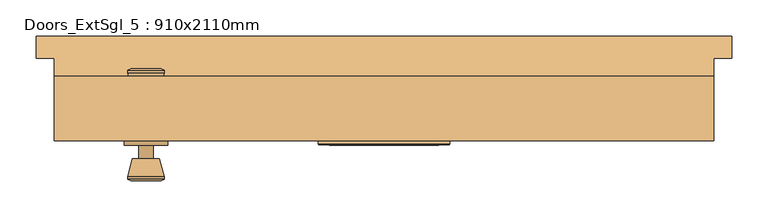
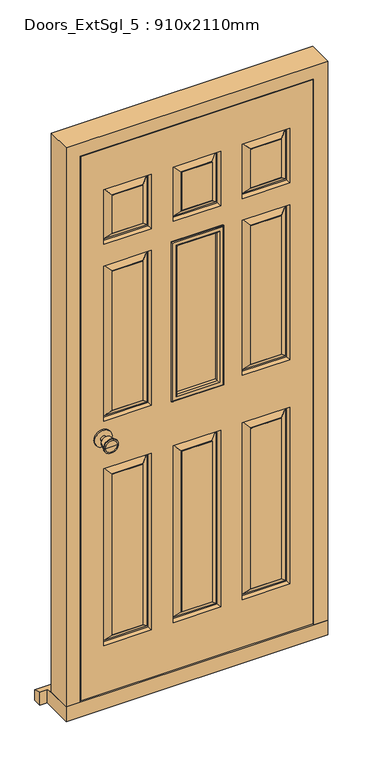
"""IFC4 building model written with IfcOpenShell, lengths in millimetres: door geometry, Doors_ExtSgl_5 : 910x2110mm."""

from ifc_helpers import new_model, si_unit, point, frame, frame_2d, origin, place, context, project, spatial, polyline, circle_curve, ellipse_curve, trimmed, segment, composite_curve, outline, extrude, faceted_brep, source, transform, mapped, element, save
from ifc_brep_helpers import plane_surface, cylinder_surface, revolved_surface, advanced_brep


def doors_extsgl_5_910x2110mm_d3ca6061(model_context):
    return source(origin(), model_context, "Body", "SolidModel", [
        advanced_brep(
        [(-328.4666667, -18.4, 1000.0), (-318.4666667, -18.4, 1000.0), (-338.4666667, -18.4, 1000.0), (-307.9907991, -67.4, 1000.0), (-328.4666667, -67.4, 1000.0), (-348.9425342, -67.4, 1000.0), (-303.4666667, -65.5721319, 1000.0), (-353.4666667, -65.5721319, 1000.0), (-303.4666667, -62.1084537, 1000.0), (-353.4666667, -62.1084537, 1000.0), (-309.8304306, -37.4, 1000.0), (-347.1029027, -37.4, 1000.0), (-318.4666667, -37.4, 1000.0), (-338.4666667, -37.4, 1000.0)],
        [
            (0, 1),
            (1, 2, circle_curve(frame((-328.4666667, -18.4, 1000.0), z_axis=(0.0, 1.0, 0.0), x_axis=(-1.0, 0.0, 0.0)), 10.0)),
            (2, 0),
            (2, 1, circle_curve(frame((-328.4666667, -18.4, 1000.0), z_axis=(0.0, 1.0, 0.0), x_axis=(-1.0, 0.0, 0.0)), 10.0)),
            (3, 4),
            (4, 5),
            (5, 3, circle_curve(frame((-328.4666667, -67.4, 1000.0), z_axis=(0.0, -1.0, 0.0), x_axis=(-1.0, 0.0, 0.0)), 20.4758676)),
            (3, 5, circle_curve(frame((-328.4666667, -67.4, 1000.0), z_axis=(0.0, -1.0, 0.0), x_axis=(-1.0, 0.0, 0.0)), 20.4758676)),
            (6, 3),
            (5, 7),
            (7, 6, circle_curve(frame((-328.4666667, -65.5721319, 1000.0), z_axis=(0.0, -1.0, 0.0), x_axis=(-1.0, 0.0, 0.0)), 25.0)),
            (6, 7, circle_curve(frame((-328.4666667, -65.5721319, 1000.0), z_axis=(0.0, -1.0, 0.0), x_axis=(-1.0, 0.0, 0.0)), 25.0)),
            (8, 6),
            (7, 9),
            (9, 8, circle_curve(frame((-328.4666667, -62.1084537, 1000.0), z_axis=(0.0, -1.0, 0.0), x_axis=(-1.0, 0.0, 0.0)), 25.0)),
            (8, 9, circle_curve(frame((-328.4666667, -62.1084537, 1000.0), z_axis=(0.0, -1.0, 0.0), x_axis=(-1.0, 0.0, 0.0)), 25.0)),
            (10, 8),
            (9, 11),
            (11, 10, circle_curve(frame((-328.4666667, -37.4, 1000.0), z_axis=(0.0, -1.0, 0.0), x_axis=(-1.0, 0.0, 0.0)), 18.636236)),
            (10, 11, circle_curve(frame((-328.4666667, -37.4, 1000.0), z_axis=(0.0, -1.0, 0.0), x_axis=(-1.0, 0.0, 0.0)), 18.636236)),
            (12, 10),
            (11, 13),
            (13, 12, circle_curve(frame((-328.4666667, -37.4, 1000.0), z_axis=(0.0, -1.0, 0.0), x_axis=(-1.0, 0.0, 0.0)), 10.0)),
            (12, 13, circle_curve(frame((-328.4666667, -37.4, 1000.0), z_axis=(0.0, -1.0, 0.0), x_axis=(-1.0, 0.0, 0.0)), 10.0)),
            (1, 12),
            (13, 2),
        ],
        [
            plane_surface(frame((-328.4666667, -18.4, 1000.0), z_axis=(0.0, 1.0, 0.0), x_axis=(-1.0, 0.0, 0.0))),
            plane_surface(frame((-328.4666667, -67.4, 1000.0), z_axis=(0.0, -1.0, 0.0), x_axis=(-1.0, 0.0, 0.0))),
            revolved_surface(polyline([(-348.9425342, -67.4, 1000.0), (-353.4666667, -65.5721319, 1000.0)]), (-328.4666667, -18.4, 1000.0), (0.0, 1.0, 0.0)),
            cylinder_surface(frame((-328.4666667, -18.4, 1000.0), z_axis=(0.0, 1.0, 0.0), x_axis=(-1.0, 0.0, 0.0)), 25.0),
            revolved_surface(polyline([(-353.4666667, -62.1084537, 1000.0), (-347.1029027, -37.4, 1000.0)]), (-328.4666667, -18.4, 1000.0), (0.0, 1.0, 0.0)),
            plane_surface(frame((-328.4666667, -37.4, 1000.0), z_axis=(0.0, 1.0, 0.0), x_axis=(-1.0, 0.0, 0.0))),
            cylinder_surface(frame((-328.4666667, -18.4, 1000.0), z_axis=(0.0, 1.0, 0.0), x_axis=(-1.0, 0.0, 0.0)), 10.0),
        ],
        [
            (0, [[1, 2, 3]]),
            (0, [[-3, 4, -1]]),
            (1, [[5, 6, 7]]),
            (1, [[-6, -5, 8]]),
            (2, [[9, -7, 10, 11]]),
            (2, [[-10, -8, -9, 12]]),
            (3, [[13, -11, 14, 15]]),
            (3, [[-14, -12, -13, 16]]),
            (4, [[17, -15, 18, 19]]),
            (4, [[-18, -16, -17, 20]]),
            (5, [[21, -19, 22, 23]]),
            (5, [[-22, -20, -21, 24]]),
            (6, [[25, -23, 26, -2]]),
            (6, [[-26, -24, -25, -4]]),
        ],
    ),
        extrude(outline(composite_curve([segment(trimmed(circle_curve(frame_2d((1000.0, -328.4666667)), 30.0), [point((1000.0, -358.4666667))], [point((1000.0, -298.4666667))], False, "CARTESIAN"), True, "CONTINUOUS"), segment(trimmed(circle_curve(frame_2d((1000.0, -328.4666667)), 30.0), [point((1000.0, -298.4666667))], [point((1000.0, -358.4666667))], False, "CARTESIAN"), True, "CONTINUOUS")], self_intersect=False)), frame((0.0, -18.4, 0.0), z_axis=(0.0, 1.0, 0.0), x_axis=(0.0, 0.0, 1.0)), (0.0, 0.0, 1.0), 6.0),
        advanced_brep(
        [(-328.4666667, 37.6, 1000.0), (-338.4666667, 37.6, 1000.0), (-318.4666667, 37.6, 1000.0), (-307.9907991, 86.6, 1000.0), (-348.9425342, 86.6, 1000.0), (-328.4666667, 86.6, 1000.0), (-303.4666667, 84.7721319, 1000.0), (-353.4666667, 84.7721319, 1000.0), (-303.4666667, 81.3084537, 1000.0), (-353.4666667, 81.3084537, 1000.0), (-309.8304306, 56.6, 1000.0), (-347.1029027, 56.6, 1000.0), (-318.4666667, 56.6, 1000.0), (-338.4666667, 56.6, 1000.0)],
        [
            (0, 1),
            (1, 2, circle_curve(frame((-328.4666667, 37.6, 1000.0), z_axis=(0.0, -1.0, 0.0), x_axis=(-1.0, 0.0, 0.0)), 10.0)),
            (2, 0),
            (2, 1, circle_curve(frame((-328.4666667, 37.6, 1000.0), z_axis=(0.0, -1.0, 0.0), x_axis=(-1.0, 0.0, 0.0)), 10.0)),
            (3, 4, circle_curve(frame((-328.4666667, 86.6, 1000.0), z_axis=(0.0, 1.0, 0.0), x_axis=(-1.0, 0.0, 0.0)), 20.4758676)),
            (4, 5),
            (5, 3),
            (4, 3, circle_curve(frame((-328.4666667, 86.6, 1000.0), z_axis=(0.0, 1.0, 0.0), x_axis=(-1.0, 0.0, 0.0)), 20.4758676)),
            (6, 7, circle_curve(frame((-328.4666667, 84.7721319, 1000.0), z_axis=(0.0, 1.0, 0.0), x_axis=(-1.0, 0.0, 0.0)), 25.0)),
            (7, 4),
            (3, 6),
            (7, 6, circle_curve(frame((-328.4666667, 84.7721319, 1000.0), z_axis=(0.0, 1.0, 0.0), x_axis=(-1.0, 0.0, 0.0)), 25.0)),
            (8, 9, circle_curve(frame((-328.4666667, 81.3084537, 1000.0), z_axis=(0.0, 1.0, 0.0), x_axis=(-1.0, 0.0, 0.0)), 25.0)),
            (9, 7),
            (6, 8),
            (9, 8, circle_curve(frame((-328.4666667, 81.3084537, 1000.0), z_axis=(0.0, 1.0, 0.0), x_axis=(-1.0, 0.0, 0.0)), 25.0)),
            (10, 11, circle_curve(frame((-328.4666667, 56.6, 1000.0), z_axis=(0.0, 1.0, 0.0), x_axis=(-1.0, 0.0, 0.0)), 18.636236)),
            (11, 9),
            (8, 10),
            (11, 10, circle_curve(frame((-328.4666667, 56.6, 1000.0), z_axis=(0.0, 1.0, 0.0), x_axis=(-1.0, 0.0, 0.0)), 18.636236)),
            (12, 13, circle_curve(frame((-328.4666667, 56.6, 1000.0), z_axis=(0.0, 1.0, 0.0), x_axis=(-1.0, 0.0, 0.0)), 10.0)),
            (13, 11),
            (10, 12),
            (13, 12, circle_curve(frame((-328.4666667, 56.6, 1000.0), z_axis=(0.0, 1.0, 0.0), x_axis=(-1.0, 0.0, 0.0)), 10.0)),
            (1, 13),
            (12, 2),
        ],
        [
            plane_surface(frame((-328.4666667, 37.6, 1000.0), z_axis=(0.0, -1.0, 0.0), x_axis=(-1.0, 0.0, 0.0))),
            plane_surface(frame((-328.4666667, 86.6, 1000.0), z_axis=(0.0, 1.0, 0.0), x_axis=(-1.0, 0.0, 0.0))),
            revolved_surface(polyline([(-348.9425342, 86.6, 1000.0), (-353.4666667, 84.7721319, 1000.0)]), (-328.4666667, 37.6, 1000.0), (0.0, -1.0, 0.0)),
            cylinder_surface(frame((-328.4666667, 37.6, 1000.0), z_axis=(0.0, -1.0, 0.0), x_axis=(-1.0, 0.0, 0.0)), 25.0),
            revolved_surface(polyline([(-353.4666667, 81.3084537, 1000.0), (-347.1029027, 56.6, 1000.0)]), (-328.4666667, 37.6, 1000.0), (0.0, -1.0, 0.0)),
            plane_surface(frame((-328.4666667, 56.6, 1000.0), z_axis=(0.0, -1.0, 0.0), x_axis=(-1.0, 0.0, 0.0))),
            cylinder_surface(frame((-328.4666667, 37.6, 1000.0), z_axis=(0.0, -1.0, 0.0), x_axis=(-1.0, 0.0, 0.0)), 10.0),
        ],
        [
            (0, [[1, 2, 3]]),
            (0, [[-3, 4, -1]]),
            (1, [[5, 6, 7]]),
            (1, [[8, -7, -6]]),
            (2, [[9, 10, -5, 11]]),
            (2, [[12, -11, -8, -10]]),
            (3, [[13, 14, -9, 15]]),
            (3, [[16, -15, -12, -14]]),
            (4, [[17, 18, -13, 19]]),
            (4, [[20, -19, -16, -18]]),
            (5, [[21, 22, -17, 23]]),
            (5, [[24, -23, -20, -22]]),
            (6, [[-2, 25, -21, 26]]),
            (6, [[-4, -26, -24, -25]]),
        ],
    ),
        extrude(outline(composite_curve([segment(trimmed(circle_curve(frame_2d((1000.0, -328.4666667)), 30.0), [point((1000.0, -358.4666667))], [point((1000.0, -298.4666667))], False, "CARTESIAN"), True, "CONTINUOUS"), segment(trimmed(circle_curve(frame_2d((1000.0, -328.4666667)), 30.0), [point((1000.0, -298.4666667))], [point((1000.0, -358.4666667))], False, "CARTESIAN"), True, "CONTINUOUS")], self_intersect=False)), frame((0.0, 31.6, 0.0), z_axis=(0.0, 1.0, 0.0), x_axis=(0.0, 0.0, 1.0)), (0.0, 0.0, 1.0), 6.0),
        faceted_brep([(384.5333333, 76.6, 54.5), (455.0333333, 76.6, 54.5), (455.0333333, -12.4, 54.5), (406.5333333, -12.4, 54.5), (406.5333333, 34.6, 54.5), (384.5333333, 34.6, 54.5), (384.5333333, 76.6, 2039.5), (-384.4666667, 76.6, 2039.5), (-384.4666667, 76.6, 54.5), (-454.9666667, 76.6, 54.5), (-454.9666667, 76.6, 2110.0), (455.0333333, 76.6, 2110.0), (455.0333333, -12.4, 2110.0), (-454.9666667, -12.4, 2110.0), (-454.9666667, -12.4, 54.5), (-406.4666667, -12.4, 54.5), (-406.4666667, -12.4, 2061.5), (406.5333333, -12.4, 2061.5), (406.5333333, 34.6, 2061.5), (-406.4666667, 34.6, 2061.5), (-406.4666667, 34.6, 54.5), (-384.4666667, 34.6, 54.5), (-384.4666667, 34.6, 2039.5), (384.5333333, 34.6, 2039.5)], [[[0, 1, 2, 3, 4, 5]], [[1, 0, 6, 7, 8, 9, 10, 11]], [[2, 1, 11, 12]], [[3, 2, 12, 13, 14, 15, 16, 17]], [[4, 3, 17, 18]], [[5, 4, 18, 19, 20, 21, 22, 23]], [[0, 5, 23, 6]], [[8, 7, 22, 21]], [[9, 8, 21, 20, 15, 14]], [[10, 9, 14, 13]], [[16, 15, 20, 19]], [[11, 10, 13, 12]], [[17, 16, 19, 18]], [[7, 6, 23, 22]]]),
        faceted_brep([(403.5333333, -12.4, 58.5), (403.5333333, -12.4, 2058.5), (-404.3916961, -12.4, 2058.5), (-404.3916961, -12.4, 58.5), (-82.8, -12.4, 1058.5), (-82.8, -12.4, 1628.5), (82.8666667, -12.4, 1628.5), (82.8666667, -12.4, 1058.5), (-157.8, -12.4, 883.5), (-157.8, -12.4, 233.5), (-323.4666667, -12.4, 233.5), (-323.4666667, -12.4, 883.5), (323.5333333, -12.4, 883.5), (323.5333333, -12.4, 233.5), (157.8666667, -12.4, 233.5), (157.8666667, -12.4, 883.5), (82.8666667, -12.4, 883.5), (82.8666667, -12.4, 233.5), (-82.8, -12.4, 233.5), (-82.8, -12.4, 883.5), (-323.4666667, -12.4, 1058.5), (-323.4666667, -12.4, 1628.5), (-157.8, -12.4, 1628.5), (-157.8, -12.4, 1058.5), (323.5333333, -12.4, 1628.5), (323.5333333, -12.4, 1058.5), (157.8666667, -12.4, 1058.5), (157.8666667, -12.4, 1628.5), (-157.8, -12.4, 1908.5), (-157.8, -12.4, 1708.5), (-323.4666667, -12.4, 1708.5), (-323.4666667, -12.4, 1908.5), (82.8666667, -12.4, 1908.5), (82.8666667, -12.4, 1708.5), (-82.8, -12.4, 1708.5), (-82.8, -12.4, 1908.5), (323.5333333, -12.4, 1908.5), (323.5333333, -12.4, 1708.5), (157.8666667, -12.4, 1708.5), (157.8666667, -12.4, 1908.5), (-187.8, -12.4, 263.5), (-187.8, -12.4, 853.5), (-293.4666667, -12.4, 853.5), (-293.4666667, -12.4, 263.5), (293.5333333, -12.4, 263.5), (293.5333333, -12.4, 853.5), (187.8666667, -12.4, 853.5), (187.8666667, -12.4, 263.5), (52.8666667, -12.4, 263.5), (52.8666667, -12.4, 853.5), (-52.8, -12.4, 853.5), (-52.8, -12.4, 263.5), (-293.4666667, -12.4, 1598.5), (-293.4666667, -12.4, 1088.5), (-187.8, -12.4, 1088.5), (-187.8, -12.4, 1598.5), (293.5333333, -12.4, 1088.5), (293.5333333, -12.4, 1598.5), (187.8666667, -12.4, 1598.5), (187.8666667, -12.4, 1088.5), (-187.8, -12.4, 1738.5), (-187.8, -12.4, 1878.5), (-293.4666667, -12.4, 1878.5), (-293.4666667, -12.4, 1738.5), (52.8666667, -12.4, 1738.5), (52.8666667, -12.4, 1878.5), (-52.8, -12.4, 1878.5), (-52.8, -12.4, 1738.5), (293.5333333, -12.4, 1738.5), (293.5333333, -12.4, 1878.5), (187.8666667, -12.4, 1878.5), (187.8666667, -12.4, 1738.5), (403.5333333, 31.6, 58.5), (-404.3916961, 31.6, 58.5), (-404.3916961, 31.6, 2058.5), (403.5333333, 31.6, 2058.5), (-82.8, 31.6, 1058.5), (82.8666667, 31.6, 1058.5), (82.8666667, 31.6, 1628.5), (-82.8, 31.6, 1628.5), (157.8666667, 31.6, 883.5), (157.8666667, 31.6, 233.5), (323.5333333, 31.6, 233.5), (323.5333333, 31.6, 883.5), (-323.4666667, 31.6, 883.5), (-323.4666667, 31.6, 233.5), (-157.8, 31.6, 233.5), (-157.8, 31.6, 883.5), (-82.8, 31.6, 883.5), (-82.8, 31.6, 233.5), (82.8666667, 31.6, 233.5), (82.8666667, 31.6, 883.5), (157.8666667, 31.6, 1628.5), (157.8666667, 31.6, 1058.5), (323.5333333, 31.6, 1058.5), (323.5333333, 31.6, 1628.5), (-323.4666667, 31.6, 1628.5), (-323.4666667, 31.6, 1058.5), (-157.8, 31.6, 1058.5), (-157.8, 31.6, 1628.5), (323.5333333, 31.6, 1708.5), (323.5333333, 31.6, 1908.5), (157.8666667, 31.6, 1908.5), (157.8666667, 31.6, 1708.5), (-82.8, 31.6, 1908.5), (-82.8, 31.6, 1708.5), (82.8666667, 31.6, 1708.5), (82.8666667, 31.6, 1908.5), (-323.4666667, 31.6, 1908.5), (-323.4666667, 31.6, 1708.5), (-157.8, 31.6, 1708.5), (-157.8, 31.6, 1908.5), (187.8666667, 31.6, 263.5), (187.8666667, 31.6, 853.5), (293.5333333, 31.6, 853.5), (293.5333333, 31.6, 263.5), (-293.4666667, 31.6, 263.5), (-293.4666667, 31.6, 853.5), (-187.8, 31.6, 853.5), (-187.8, 31.6, 263.5), (-52.8, 31.6, 263.5), (-52.8, 31.6, 853.5), (52.8666667, 31.6, 853.5), (52.8666667, 31.6, 263.5), (187.8666667, 31.6, 1088.5), (187.8666667, 31.6, 1598.5), (293.5333333, 31.6, 1598.5), (293.5333333, 31.6, 1088.5), (-293.4666667, 31.6, 1088.5), (-293.4666667, 31.6, 1598.5), (-187.8, 31.6, 1598.5), (-187.8, 31.6, 1088.5), (293.5333333, 31.6, 1878.5), (293.5333333, 31.6, 1738.5), (187.8666667, 31.6, 1738.5), (187.8666667, 31.6, 1878.5), (-52.8, 31.6, 1738.5), (-52.8, 31.6, 1878.5), (52.8666667, 31.6, 1878.5), (52.8666667, 31.6, 1738.5), (-293.4666667, 31.6, 1738.5), (-293.4666667, 31.6, 1878.5), (-187.8, 31.6, 1878.5), (-187.8, 31.6, 1738.5), (160.8666667, 16.6, 880.5), (160.8666667, 16.6, 236.5), (185.8666667, 30.6, 855.5), (185.8666667, 30.6, 261.5), (165.8666667, 16.6, 241.5), (165.8666667, 16.6, 875.5), (187.8666667, 30.6, 263.5), (187.8666667, 30.6, 853.5), (320.5333333, 16.6, 236.5), (295.5333333, 30.6, 261.5), (315.5333333, 16.6, 241.5), (293.5333333, 30.6, 263.5), (320.5333333, 16.6, 880.5), (295.5333333, 30.6, 855.5), (315.5333333, 16.6, 875.5), (293.5333333, 30.6, 853.5), (-320.4666667, 16.6, 880.5), (-320.4666667, 16.6, 236.5), (-295.4666667, 30.6, 855.5), (-295.4666667, 30.6, 261.5), (-315.4666667, 16.6, 241.5), (-315.4666667, 16.6, 875.5), (-293.4666667, 30.6, 263.5), (-293.4666667, 30.6, 853.5), (-160.8, 16.6, 236.5), (-185.8, 30.6, 261.5), (-165.8, 16.6, 241.5), (-187.8, 30.6, 263.5), (-160.8, 16.6, 880.5), (-185.8, 30.6, 855.5), (-165.8, 16.6, 875.5), (-187.8, 30.6, 853.5), (-187.8, -11.4, 263.5), (-187.8, -11.4, 853.5), (-165.8, 2.6, 241.5), (-165.8, 2.6, 875.5), (-185.8, -11.4, 855.5), (-185.8, -11.4, 261.5), (-160.8, 2.6, 880.5), (-160.8, 2.6, 236.5), (-293.4666667, -11.4, 853.5), (-315.4666667, 2.6, 875.5), (-295.4666667, -11.4, 855.5), (-320.4666667, 2.6, 880.5), (-293.4666667, -11.4, 263.5), (-315.4666667, 2.6, 241.5), (-295.4666667, -11.4, 261.5), (-320.4666667, 2.6, 236.5), (320.5333333, 2.6, 880.5), (320.5333333, 2.6, 236.5), (295.5333333, -11.4, 855.5), (295.5333333, -11.4, 261.5), (315.5333333, 2.6, 241.5), (315.5333333, 2.6, 875.5), (293.5333333, -11.4, 263.5), (293.5333333, -11.4, 853.5), (160.8666667, 2.6, 236.5), (185.8666667, -11.4, 261.5), (165.8666667, 2.6, 241.5), (187.8666667, -11.4, 263.5), (160.8666667, 2.6, 880.5), (185.8666667, -11.4, 855.5), (165.8666667, 2.6, 875.5), (187.8666667, -11.4, 853.5), (-52.8, 30.6, 263.5), (-52.8, 30.6, 853.5), (-74.8, 16.6, 241.5), (-74.8, 16.6, 875.5), (-54.8, 30.6, 855.5), (-54.8, 30.6, 261.5), (-79.8, 16.6, 880.5), (-79.8, 16.6, 236.5), (52.8666667, 30.6, 853.5), (74.8666667, 16.6, 875.5), (54.8666667, 30.6, 855.5), (79.8666667, 16.6, 880.5), (52.8666667, 30.6, 263.5), (74.8666667, 16.6, 241.5), (54.8666667, 30.6, 261.5), (79.8666667, 16.6, 236.5), (79.8666667, 2.6, 880.5), (79.8666667, 2.6, 236.5), (54.8666667, -11.4, 855.5), (54.8666667, -11.4, 261.5), (74.8666667, 2.6, 241.5), (74.8666667, 2.6, 875.5), (52.8666667, -11.4, 263.5), (52.8666667, -11.4, 853.5), (-79.8, 2.6, 236.5), (-54.8, -11.4, 261.5), (-74.8, 2.6, 241.5), (-52.8, -11.4, 263.5), (-79.8, 2.6, 880.5), (-54.8, -11.4, 855.5), (-74.8, 2.6, 875.5), (-52.8, -11.4, 853.5), (187.8666667, 30.6, 1088.5), (187.8666667, 30.6, 1598.5), (165.8666667, 16.6, 1066.5), (165.8666667, 16.6, 1620.5), (185.8666667, 30.6, 1600.5), (185.8666667, 30.6, 1086.5), (160.8666667, 16.6, 1625.5), (160.8666667, 16.6, 1061.5), (293.5333333, 30.6, 1598.5), (315.5333333, 16.6, 1620.5), (295.5333333, 30.6, 1600.5), (320.5333333, 16.6, 1625.5), (293.5333333, 30.6, 1088.5), (315.5333333, 16.6, 1066.5), (295.5333333, 30.6, 1086.5), (320.5333333, 16.6, 1061.5), (-293.4666667, 30.6, 1088.5), (-293.4666667, 30.6, 1598.5), (-315.4666667, 16.6, 1066.5), (-315.4666667, 16.6, 1620.5), (-295.4666667, 30.6, 1600.5), (-295.4666667, 30.6, 1086.5), (-320.4666667, 16.6, 1625.5), (-320.4666667, 16.6, 1061.5), (-187.8, 30.6, 1598.5), (-165.8, 16.6, 1620.5), (-185.8, 30.6, 1600.5), (-160.8, 16.6, 1625.5), (-187.8, 30.6, 1088.5), (-165.8, 16.6, 1066.5), (-185.8, 30.6, 1086.5), (-160.8, 16.6, 1061.5), (293.5333333, 30.6, 1878.5), (293.5333333, 30.6, 1738.5), (315.5333333, 16.6, 1900.5), (315.5333333, 16.6, 1716.5), (295.5333333, 30.6, 1736.5), (295.5333333, 30.6, 1880.5), (320.5333333, 16.6, 1711.5), (320.5333333, 16.6, 1905.5), (187.8666667, 30.6, 1738.5), (165.8666667, 16.6, 1716.5), (185.8666667, 30.6, 1736.5), (160.8666667, 16.6, 1711.5), (187.8666667, 30.6, 1878.5), (165.8666667, 16.6, 1900.5), (185.8666667, 30.6, 1880.5), (160.8666667, 16.6, 1905.5), (-52.8, 30.6, 1738.5), (-52.8, 30.6, 1878.5), (-74.8, 16.6, 1716.5), (-74.8, 16.6, 1900.5), (-54.8, 30.6, 1880.5), (-54.8, 30.6, 1736.5), (-79.8, 16.6, 1905.5), (-79.8, 16.6, 1711.5), (52.8666667, 30.6, 1878.5), (74.8666667, 16.6, 1900.5), (54.8666667, 30.6, 1880.5), (79.8666667, 16.6, 1905.5), (52.8666667, 30.6, 1738.5), (74.8666667, 16.6, 1716.5), (54.8666667, 30.6, 1736.5), (79.8666667, 16.6, 1711.5), (-293.4666667, 30.6, 1738.5), (-293.4666667, 30.6, 1878.5), (-315.4666667, 16.6, 1716.5), (-315.4666667, 16.6, 1900.5), (-295.4666667, 30.6, 1880.5), (-295.4666667, 30.6, 1736.5), (-320.4666667, 16.6, 1905.5), (-320.4666667, 16.6, 1711.5), (-187.8, 30.6, 1878.5), (-165.8, 16.6, 1900.5), (-185.8, 30.6, 1880.5), (-160.8, 16.6, 1905.5), (-187.8, 30.6, 1738.5), (-165.8, 16.6, 1716.5), (-185.8, 30.6, 1736.5), (-160.8, 16.6, 1711.5), (-320.4666667, 2.6, 1061.5), (-320.4666667, 2.6, 1625.5), (-295.4666667, -11.4, 1086.5), (-295.4666667, -11.4, 1600.5), (-315.4666667, 2.6, 1620.5), (-315.4666667, 2.6, 1066.5), (-293.4666667, -11.4, 1598.5), (-293.4666667, -11.4, 1088.5), (-160.8, 2.6, 1625.5), (-185.8, -11.4, 1600.5), (-165.8, 2.6, 1620.5), (-187.8, -11.4, 1598.5), (-160.8, 2.6, 1061.5), (-185.8, -11.4, 1086.5), (-165.8, 2.6, 1066.5), (-187.8, -11.4, 1088.5), (320.5333333, 2.6, 1625.5), (320.5333333, 2.6, 1061.5), (295.5333333, -11.4, 1600.5), (295.5333333, -11.4, 1086.5), (315.5333333, 2.6, 1066.5), (315.5333333, 2.6, 1620.5), (293.5333333, -11.4, 1088.5), (293.5333333, -11.4, 1598.5), (160.8666667, 2.6, 1061.5), (185.8666667, -11.4, 1086.5), (165.8666667, 2.6, 1066.5), (187.8666667, -11.4, 1088.5), (160.8666667, 2.6, 1625.5), (185.8666667, -11.4, 1600.5), (165.8666667, 2.6, 1620.5), (187.8666667, -11.4, 1598.5), (-187.8, -11.4, 1738.5), (-187.8, -11.4, 1878.5), (-165.8, 2.6, 1716.5), (-165.8, 2.6, 1900.5), (-185.8, -11.4, 1880.5), (-185.8, -11.4, 1736.5), (-160.8, 2.6, 1905.5), (-160.8, 2.6, 1711.5), (-293.4666667, -11.4, 1878.5), (-315.4666667, 2.6, 1900.5), (-295.4666667, -11.4, 1880.5), (-320.4666667, 2.6, 1905.5), (-293.4666667, -11.4, 1738.5), (-315.4666667, 2.6, 1716.5), (-295.4666667, -11.4, 1736.5), (-320.4666667, 2.6, 1711.5), (52.8666667, -11.4, 1738.5), (52.8666667, -11.4, 1878.5), (74.8666667, 2.6, 1716.5), (74.8666667, 2.6, 1900.5), (54.8666667, -11.4, 1880.5), (54.8666667, -11.4, 1736.5), (79.8666667, 2.6, 1905.5), (79.8666667, 2.6, 1711.5), (-52.8, -11.4, 1878.5), (-74.8, 2.6, 1900.5), (-54.8, -11.4, 1880.5), (-79.8, 2.6, 1905.5), (-52.8, -11.4, 1738.5), (-74.8, 2.6, 1716.5), (-54.8, -11.4, 1736.5), (-79.8, 2.6, 1711.5), (293.5333333, -11.4, 1738.5), (293.5333333, -11.4, 1878.5), (315.5333333, 2.6, 1716.5), (315.5333333, 2.6, 1900.5), (295.5333333, -11.4, 1880.5), (295.5333333, -11.4, 1736.5), (320.5333333, 2.6, 1905.5), (320.5333333, 2.6, 1711.5), (187.8666667, -11.4, 1878.5), (165.8666667, 2.6, 1900.5), (185.8666667, -11.4, 1880.5), (160.8666667, 2.6, 1905.5), (187.8666667, -11.4, 1738.5), (165.8666667, 2.6, 1716.5), (185.8666667, -11.4, 1736.5), (160.8666667, 2.6, 1711.5)], [[[0, 1, 2, 3], [4, 5, 6, 7], [8, 9, 10, 11], [12, 13, 14, 15], [16, 17, 18, 19], [20, 21, 22, 23], [24, 25, 26, 27], [28, 29, 30, 31], [32, 33, 34, 35], [36, 37, 38, 39]], [[40, 41, 42, 43]], [[44, 45, 46, 47]], [[48, 49, 50, 51]], [[52, 53, 54, 55]], [[56, 57, 58, 59]], [[60, 61, 62, 63]], [[64, 65, 66, 67]], [[68, 69, 70, 71]], [[72, 73, 74, 75], [76, 77, 78, 79], [80, 81, 82, 83], [84, 85, 86, 87], [88, 89, 90, 91], [92, 93, 94, 95], [96, 97, 98, 99], [100, 101, 102, 103], [104, 105, 106, 107], [108, 109, 110, 111]], [[112, 113, 114, 115]], [[116, 117, 118, 119]], [[120, 121, 122, 123]], [[124, 125, 126, 127]], [[128, 129, 130, 131]], [[132, 133, 134, 135]], [[136, 137, 138, 139]], [[140, 141, 142, 143]], [[1, 0, 72, 75]], [[2, 1, 75, 74]], [[3, 2, 74, 73]], [[0, 3, 73, 72]], [[5, 4, 76, 79]], [[6, 5, 79, 78]], [[7, 6, 78, 77]], [[4, 7, 77, 76]], [[144, 145, 81, 80]], [[146, 147, 148, 149]], [[112, 150, 151, 113]], [[81, 145, 152, 82]], [[148, 147, 153, 154]], [[150, 112, 115, 155]], [[82, 152, 156, 83]], [[154, 153, 157, 158]], [[155, 115, 114, 159]], [[144, 80, 83, 156]], [[145, 144, 156, 152], [149, 148, 154, 158]], [[146, 149, 158, 157]], [[147, 146, 157, 153], [151, 150, 155, 159]], [[113, 151, 159, 114]], [[160, 161, 85, 84]], [[162, 163, 164, 165]], [[116, 166, 167, 117]], [[85, 161, 168, 86]], [[164, 163, 169, 170]], [[166, 116, 119, 171]], [[86, 168, 172, 87]], [[170, 169, 173, 174]], [[171, 119, 118, 175]], [[160, 84, 87, 172]], [[161, 160, 172, 168], [165, 164, 170, 174]], [[162, 165, 174, 173]], [[163, 162, 173, 169], [167, 166, 171, 175]], [[117, 167, 175, 118]], [[176, 177, 41, 40]], [[178, 179, 180, 181]], [[8, 182, 183, 9]], [[41, 177, 184, 42]], [[180, 179, 185, 186]], [[182, 8, 11, 187]], [[42, 184, 188, 43]], [[186, 185, 189, 190]], [[187, 11, 10, 191]], [[176, 40, 43, 188]], [[181, 180, 186, 190], [177, 176, 188, 184]], [[178, 181, 190, 189]], [[183, 182, 187, 191], [179, 178, 189, 185]], [[9, 183, 191, 10]], [[192, 193, 13, 12]], [[194, 195, 196, 197]], [[44, 198, 199, 45]], [[13, 193, 200, 14]], [[196, 195, 201, 202]], [[198, 44, 47, 203]], [[14, 200, 204, 15]], [[202, 201, 205, 206]], [[203, 47, 46, 207]], [[192, 12, 15, 204]], [[193, 192, 204, 200], [197, 196, 202, 206]], [[194, 197, 206, 205]], [[195, 194, 205, 201], [199, 198, 203, 207]], [[45, 199, 207, 46]], [[208, 209, 121, 120]], [[210, 211, 212, 213]], [[88, 214, 215, 89]], [[121, 209, 216, 122]], [[212, 211, 217, 218]], [[214, 88, 91, 219]], [[122, 216, 220, 123]], [[218, 217, 221, 222]], [[219, 91, 90, 223]], [[208, 120, 123, 220]], [[213, 212, 218, 222], [209, 208, 220, 216]], [[210, 213, 222, 221]], [[215, 214, 219, 223], [211, 210, 221, 217]], [[89, 215, 223, 90]], [[224, 225, 17, 16]], [[226, 227, 228, 229]], [[48, 230, 231, 49]], [[17, 225, 232, 18]], [[228, 227, 233, 234]], [[230, 48, 51, 235]], [[18, 232, 236, 19]], [[234, 233, 237, 238]], [[235, 51, 50, 239]], [[224, 16, 19, 236]], [[225, 224, 236, 232], [229, 228, 234, 238]], [[226, 229, 238, 237]], [[227, 226, 237, 233], [231, 230, 235, 239]], [[49, 231, 239, 50]], [[240, 241, 125, 124]], [[242, 243, 244, 245]], [[92, 246, 247, 93]], [[125, 241, 248, 126]], [[244, 243, 249, 250]], [[246, 92, 95, 251]], [[126, 248, 252, 127]], [[250, 249, 253, 254]], [[251, 95, 94, 255]], [[240, 124, 127, 252]], [[245, 244, 250, 254], [241, 240, 252, 248]], [[242, 245, 254, 253]], [[247, 246, 251, 255], [243, 242, 253, 249]], [[93, 247, 255, 94]], [[256, 257, 129, 128]], [[258, 259, 260, 261]], [[96, 262, 263, 97]], [[129, 257, 264, 130]], [[260, 259, 265, 266]], [[262, 96, 99, 267]], [[130, 264, 268, 131]], [[266, 265, 269, 270]], [[267, 99, 98, 271]], [[256, 128, 131, 268]], [[261, 260, 266, 270], [257, 256, 268, 264]], [[258, 261, 270, 269]], [[263, 262, 267, 271], [259, 258, 269, 265]], [[97, 263, 271, 98]], [[272, 273, 133, 132]], [[274, 275, 276, 277]], [[100, 278, 279, 101]], [[133, 273, 280, 134]], [[276, 275, 281, 282]], [[278, 100, 103, 283]], [[134, 280, 284, 135]], [[282, 281, 285, 286]], [[283, 103, 102, 287]], [[272, 132, 135, 284]], [[277, 276, 282, 286], [273, 272, 284, 280]], [[274, 277, 286, 285]], [[279, 278, 283, 287], [275, 274, 285, 281]], [[101, 279, 287, 102]], [[288, 289, 137, 136]], [[290, 291, 292, 293]], [[104, 294, 295, 105]], [[137, 289, 296, 138]], [[292, 291, 297, 298]], [[294, 104, 107, 299]], [[138, 296, 300, 139]], [[298, 297, 301, 302]], [[299, 107, 106, 303]], [[288, 136, 139, 300]], [[293, 292, 298, 302], [289, 288, 300, 296]], [[290, 293, 302, 301]], [[295, 294, 299, 303], [291, 290, 301, 297]], [[105, 295, 303, 106]], [[304, 305, 141, 140]], [[306, 307, 308, 309]], [[108, 310, 311, 109]], [[141, 305, 312, 142]], [[308, 307, 313, 314]], [[310, 108, 111, 315]], [[142, 312, 316, 143]], [[314, 313, 317, 318]], [[315, 111, 110, 319]], [[304, 140, 143, 316]], [[309, 308, 314, 318], [305, 304, 316, 312]], [[306, 309, 318, 317]], [[311, 310, 315, 319], [307, 306, 317, 313]], [[109, 311, 319, 110]], [[320, 321, 21, 20]], [[322, 323, 324, 325]], [[52, 326, 327, 53]], [[21, 321, 328, 22]], [[324, 323, 329, 330]], [[326, 52, 55, 331]], [[22, 328, 332, 23]], [[330, 329, 333, 334]], [[331, 55, 54, 335]], [[320, 20, 23, 332]], [[321, 320, 332, 328], [325, 324, 330, 334]], [[322, 325, 334, 333]], [[323, 322, 333, 329], [327, 326, 331, 335]], [[53, 327, 335, 54]], [[336, 337, 25, 24]], [[338, 339, 340, 341]], [[56, 342, 343, 57]], [[25, 337, 344, 26]], [[340, 339, 345, 346]], [[342, 56, 59, 347]], [[26, 344, 348, 27]], [[346, 345, 349, 350]], [[347, 59, 58, 351]], [[336, 24, 27, 348]], [[337, 336, 348, 344], [341, 340, 346, 350]], [[338, 341, 350, 349]], [[339, 338, 349, 345], [343, 342, 347, 351]], [[57, 343, 351, 58]], [[352, 353, 61, 60]], [[354, 355, 356, 357]], [[28, 358, 359, 29]], [[61, 353, 360, 62]], [[356, 355, 361, 362]], [[358, 28, 31, 363]], [[62, 360, 364, 63]], [[362, 361, 365, 366]], [[363, 31, 30, 367]], [[352, 60, 63, 364]], [[357, 356, 362, 366], [353, 352, 364, 360]], [[354, 357, 366, 365]], [[359, 358, 363, 367], [355, 354, 365, 361]], [[29, 359, 367, 30]], [[368, 369, 65, 64]], [[370, 371, 372, 373]], [[32, 374, 375, 33]], [[65, 369, 376, 66]], [[372, 371, 377, 378]], [[374, 32, 35, 379]], [[66, 376, 380, 67]], [[378, 377, 381, 382]], [[379, 35, 34, 383]], [[368, 64, 67, 380]], [[373, 372, 378, 382], [369, 368, 380, 376]], [[370, 373, 382, 381]], [[375, 374, 379, 383], [371, 370, 381, 377]], [[33, 375, 383, 34]], [[384, 385, 69, 68]], [[386, 387, 388, 389]], [[36, 390, 391, 37]], [[69, 385, 392, 70]], [[388, 387, 393, 394]], [[390, 36, 39, 395]], [[70, 392, 396, 71]], [[394, 393, 397, 398]], [[395, 39, 38, 399]], [[384, 68, 71, 396]], [[389, 388, 394, 398], [385, 384, 396, 392]], [[386, 389, 398, 397]], [[391, 390, 395, 399], [387, 386, 397, 393]], [[37, 391, 399, 38]]]),
        faceted_brep([(480.0333333, 131.6, 0.0), (480.0333333, 131.6, 38.5947221), (480.0333333, 101.6, 47.2703282), (480.0333333, 101.6, 0.0), (-479.9666667, 131.6, 38.5947221), (-479.9666667, 131.6, 0.0), (-479.9666667, 101.6, 0.0), (-479.9666667, 101.6, 47.2703282), (455.0333333, 101.6, 0.0), (455.0333333, -12.4, 0.0), (-454.9666667, -12.4, 0.0), (-454.9666667, 101.6, 0.0), (-454.9666667, 101.6, 47.2703282), (-454.9666667, 76.6, 54.5), (455.0333333, 76.6, 54.5), (455.0333333, 101.6, 47.2703282), (-454.9666667, -12.4, 54.5), (455.0333333, -12.4, 54.5)], [[[0, 1, 2, 3]], [[4, 5, 6, 7]], [[5, 0, 3, 8, 9, 10, 11, 6]], [[1, 0, 5, 4]], [[1, 4, 7, 12, 13, 14, 15, 2]], [[13, 16, 17, 14]], [[16, 10, 9, 17]], [[12, 11, 10, 16, 13]], [[11, 12, 7, 6]], [[8, 15, 14, 17, 9]], [[15, 8, 3, 2]]]),
        extrude(outline(polyline([(82.8666667, -2.4), (-82.8, -2.4), (-82.8, 21.6), (82.8666667, 21.6), (82.8666667, -2.4)])), frame((0.0, 0.0, 1058.5), z_axis=(0.0, 0.0, 1.0), x_axis=(1.0, 0.0, 0.0)), (0.0, 0.0, 1.0), 570.0),
        advanced_brep(
        [(-90.8, 35.6, 1050.5), (-90.8, 31.6, 1050.5), (-90.8, 31.6, 1636.5), (-90.8, 35.6, 1636.5), (-88.8, 37.6, 1052.5), (-88.8, 37.6, 1634.5), (-70.8, 32.6, 1070.5), (-75.8, 37.6, 1065.5), (-75.8, 37.6, 1621.5), (-70.8, 32.6, 1616.5), (-70.8, 21.6, 1070.5), (-70.8, 21.6, 1616.5), (-82.8, 31.6, 1058.5), (-82.8, 21.6, 1058.5), (-82.8, 21.6, 1628.5), (-82.8, 31.6, 1628.5), (90.8666667, 31.6, 1636.5), (90.8666667, 35.6, 1636.5), (88.8666667, 37.6, 1634.5), (75.8666667, 37.6, 1621.5), (70.8666667, 32.6, 1616.5), (70.8666667, 21.6, 1616.5), (82.8666667, 21.6, 1628.5), (82.8666667, 31.6, 1628.5), (90.8666667, 31.6, 1050.5), (90.8666667, 35.6, 1050.5), (88.8666667, 37.6, 1052.5), (75.8666667, 37.6, 1065.5), (70.8666667, 32.6, 1070.5), (70.8666667, 21.6, 1070.5), (82.8666667, 21.6, 1058.5), (82.8666667, 31.6, 1058.5)],
        [
            (0, 1),
            (1, 2),
            (2, 3),
            (3, 0),
            (4, 0, ellipse_curve(frame((-88.8, 35.6, 1052.5), z_axis=(-0.7071067811865475, 0.0, 0.7071067811865475), x_axis=(-0.7071067811865474, 0.0, -0.7071067811865476)), 2.8284271, 2.0)),
            (3, 5, ellipse_curve(frame((-88.8, 35.6, 1634.5), z_axis=(-0.7071067811865475, 0.0, -0.7071067811865475), x_axis=(0.7071067811865474, 0.0, -0.7071067811865476)), 2.8284271, 2.0)),
            (5, 4),
            (6, 7, ellipse_curve(frame((-75.8, 32.6, 1065.5), z_axis=(-0.7071067811865475, 0.0, 0.7071067811865475), x_axis=(-0.7071067811865474, 0.0, -0.7071067811865476)), 7.0710678, 5.0)),
            (7, 8),
            (8, 9, ellipse_curve(frame((-75.8, 32.6, 1621.5), z_axis=(-0.7071067811865475, 0.0, -0.7071067811865475), x_axis=(0.7071067811865474, 0.0, -0.7071067811865476)), 7.0710678, 5.0)),
            (9, 6),
            (10, 6),
            (9, 11),
            (11, 10),
            (12, 13),
            (13, 14),
            (14, 15),
            (15, 12),
            (2, 16),
            (16, 17),
            (17, 3),
            (17, 18, ellipse_curve(frame((88.8666667, 35.6, 1634.5), z_axis=(-0.7071067811865475, 0.0, 0.7071067811865475), x_axis=(-0.7071067811865476, 0.0, -0.7071067811865474)), 2.8284271, 2.0)),
            (18, 5),
            (8, 19),
            (19, 20, ellipse_curve(frame((75.8666667, 32.6, 1621.5), z_axis=(-0.7071067811865475, 0.0, 0.7071067811865475), x_axis=(-0.7071067811865476, 0.0, -0.7071067811865474)), 7.0710678, 5.0)),
            (20, 9),
            (20, 21),
            (21, 11),
            (14, 22),
            (22, 23),
            (23, 15),
            (16, 24),
            (24, 25),
            (25, 17),
            (25, 26, ellipse_curve(frame((88.8666667, 35.6, 1052.5), z_axis=(0.7071067811865475, 0.0, 0.7071067811865475), x_axis=(-0.7071067811865474, 0.0, 0.7071067811865476)), 2.8284271, 2.0)),
            (26, 18),
            (19, 27),
            (27, 28, ellipse_curve(frame((75.8666667, 32.6, 1065.5), z_axis=(0.7071067811865475, 0.0, 0.7071067811865475), x_axis=(-0.7071067811865474, 0.0, 0.7071067811865476)), 7.0710678, 5.0)),
            (28, 20),
            (28, 29),
            (29, 21),
            (22, 30),
            (30, 31),
            (31, 23),
            (24, 1),
            (0, 25),
            (4, 26),
            (7, 27),
            (6, 28),
            (10, 29),
            (13, 30),
            (12, 31),
        ],
        [
            plane_surface(frame((-90.8, 31.6, 1050.5), z_axis=(-1.0, 0.0, 0.0), x_axis=(0.0, 0.0, 1.0))),
            cylinder_surface(frame((-88.8, 35.6, 1058.5), z_axis=(0.0, 0.0, -1.0), x_axis=(-1.0, 0.0, 0.0)), 2.0),
            cylinder_surface(frame((-75.8, 32.6, 1058.5), z_axis=(0.0, 0.0, -1.0), x_axis=(-1.0, 0.0, 0.0)), 5.0),
            plane_surface(frame((-70.8, 32.6, 1070.5), z_axis=(1.0, 0.0, 0.0), x_axis=(0.0, 0.0, 1.0))),
            plane_surface(frame((-82.8, 21.6, 1058.5), z_axis=(-1.0, 0.0, 0.0), x_axis=(0.0, 0.0, 1.0))),
            plane_surface(frame((-90.8, 31.6, 1636.5), z_axis=(0.0, 0.0, 1.0), x_axis=(1.0, 0.0, 0.0))),
            cylinder_surface(frame((-82.8, 35.6, 1634.5), z_axis=(-1.0, 0.0, 0.0), x_axis=(0.0, 0.0, 1.0)), 2.0),
            cylinder_surface(frame((-82.8, 32.6, 1621.5), z_axis=(-1.0, 0.0, 0.0), x_axis=(0.0, 0.0, 1.0)), 5.0),
            plane_surface(frame((-70.8, 32.6, 1616.5), z_axis=(0.0, 0.0, -1.0), x_axis=(1.0, 0.0, 0.0))),
            plane_surface(frame((-82.8, 21.6, 1628.5), z_axis=(0.0, 0.0, 1.0), x_axis=(1.0, 0.0, 0.0))),
            plane_surface(frame((90.8666667, 31.6, 1636.5), z_axis=(1.0, 0.0, 0.0), x_axis=(0.0, 0.0, -1.0))),
            cylinder_surface(frame((88.8666667, 35.6, 1628.5), z_axis=(0.0, 0.0, 1.0), x_axis=(1.0, 0.0, 0.0)), 2.0),
            cylinder_surface(frame((75.8666667, 32.6, 1628.5), z_axis=(0.0, 0.0, 1.0), x_axis=(1.0, 0.0, 0.0)), 5.0),
            plane_surface(frame((70.8666667, 32.6, 1616.5), z_axis=(-1.0, 0.0, 0.0), x_axis=(0.0, 0.0, -1.0))),
            plane_surface(frame((82.8666667, 21.6, 1628.5), z_axis=(1.0, 0.0, 0.0), x_axis=(0.0, 0.0, -1.0))),
            plane_surface(frame((90.8666667, 31.6, 1050.5), z_axis=(0.0, 0.0, -1.0), x_axis=(-1.0, 0.0, 0.0))),
            cylinder_surface(frame((82.8666667, 35.6, 1052.5), z_axis=(1.0, 0.0, 0.0), x_axis=(0.0, 0.0, -1.0)), 2.0),
            plane_surface(frame((88.8666667, 37.6, 1052.5), z_axis=(0.0, 1.0, 0.0), x_axis=(-1.0, 0.0, 0.0))),
            cylinder_surface(frame((82.8666667, 32.6, 1065.5), z_axis=(1.0, 0.0, 0.0), x_axis=(0.0, 0.0, -1.0)), 5.0),
            plane_surface(frame((70.8666667, 32.6, 1070.5), z_axis=(0.0, 0.0, 1.0), x_axis=(-1.0, 0.0, 0.0))),
            plane_surface(frame((70.8666667, 21.6, 1070.5), z_axis=(0.0, -1.0, 0.0), x_axis=(-1.0, 0.0, 0.0))),
            plane_surface(frame((82.8666667, 21.6, 1058.5), z_axis=(0.0, 0.0, -1.0), x_axis=(-1.0, 0.0, 0.0))),
            plane_surface(frame((82.8666667, 31.6, 1058.5), z_axis=(0.0, -1.0, 0.0), x_axis=(-1.0, 0.0, 0.0))),
        ],
        [
            (0, [[1, 2, 3, 4]]),
            (1, [[5, -4, 6, 7]]),
            (2, [[8, 9, 10, 11]]),
            (3, [[12, -11, 13, 14]]),
            (4, [[15, 16, 17, 18]]),
            (5, [[-3, 19, 20, 21]]),
            (6, [[-6, -21, 22, 23]]),
            (7, [[-10, 24, 25, 26]]),
            (8, [[-13, -26, 27, 28]]),
            (9, [[-17, 29, 30, 31]]),
            (10, [[-20, 32, 33, 34]]),
            (11, [[-22, -34, 35, 36]]),
            (12, [[-25, 37, 38, 39]]),
            (13, [[-27, -39, 40, 41]]),
            (14, [[-30, 42, 43, 44]]),
            (15, [[-33, 45, -1, 46]]),
            (16, [[-35, -46, -5, 47]]),
            (17, [[-23, -36, -47, -7], [48, -37, -24, -9]]),
            (18, [[-38, -48, -8, 49]]),
            (19, [[-40, -49, -12, 50]]),
            (20, [[51, -42, -29, -16], [-28, -41, -50, -14]]),
            (21, [[-43, -51, -15, 52]]),
            (22, [[-45, -32, -19, -2], [-31, -44, -52, -18]]),
        ],
    ),
        advanced_brep(
        [(90.8666667, -16.4, 1050.5), (90.8666667, -12.4, 1050.5), (90.8666667, -12.4, 1636.5), (90.8666667, -16.4, 1636.5), (88.8666667, -18.4, 1052.5), (88.8666667, -18.4, 1634.5), (70.8666667, -13.4, 1070.5), (75.8666667, -18.4, 1065.5), (75.8666667, -18.4, 1621.5), (70.8666667, -13.4, 1616.5), (70.8666667, -2.4, 1070.5), (70.8666667, -2.4, 1616.5), (82.8666667, -12.4, 1058.5), (82.8666667, -2.4, 1058.5), (82.8666667, -2.4, 1628.5), (82.8666667, -12.4, 1628.5), (-90.8, -12.4, 1636.5), (-90.8, -16.4, 1636.5), (-88.8, -18.4, 1634.5), (-75.8, -18.4, 1621.5), (-70.8, -13.4, 1616.5), (-70.8, -2.4, 1616.5), (-82.8, -2.4, 1628.5), (-82.8, -12.4, 1628.5), (-90.8, -12.4, 1050.5), (-90.8, -16.4, 1050.5), (-88.8, -18.4, 1052.5), (-75.8, -18.4, 1065.5), (-70.8, -13.4, 1070.5), (-70.8, -2.4, 1070.5), (-82.8, -2.4, 1058.5), (-82.8, -12.4, 1058.5)],
        [
            (0, 1),
            (1, 2),
            (2, 3),
            (3, 0),
            (4, 0, ellipse_curve(frame((88.8666667, -16.4, 1052.5), z_axis=(0.7071067811865475, 0.0, 0.7071067811865475), x_axis=(0.7071067811865474, 0.0, -0.7071067811865476)), 2.8284271, 2.0)),
            (3, 5, ellipse_curve(frame((88.8666667, -16.4, 1634.5), z_axis=(0.7071067811865475, 0.0, -0.7071067811865475), x_axis=(-0.7071067811865474, 0.0, -0.7071067811865476)), 2.8284271, 2.0)),
            (5, 4),
            (6, 7, ellipse_curve(frame((75.8666667, -13.4, 1065.5), z_axis=(0.7071067811865475, 0.0, 0.7071067811865475), x_axis=(0.7071067811865474, 0.0, -0.7071067811865476)), 7.0710678, 5.0)),
            (7, 8),
            (8, 9, ellipse_curve(frame((75.8666667, -13.4, 1621.5), z_axis=(0.7071067811865475, 0.0, -0.7071067811865475), x_axis=(-0.7071067811865474, 0.0, -0.7071067811865476)), 7.0710678, 5.0)),
            (9, 6),
            (10, 6),
            (9, 11),
            (11, 10),
            (12, 13),
            (13, 14),
            (14, 15),
            (15, 12),
            (2, 16),
            (16, 17),
            (17, 3),
            (17, 18, ellipse_curve(frame((-88.8, -16.4, 1634.5), z_axis=(0.7071067811865475, 0.0, 0.7071067811865475), x_axis=(0.7071067811865476, 0.0, -0.7071067811865474)), 2.8284271, 2.0)),
            (18, 5),
            (8, 19),
            (19, 20, ellipse_curve(frame((-75.8, -13.4, 1621.5), z_axis=(0.7071067811865475, 0.0, 0.7071067811865475), x_axis=(0.7071067811865476, 0.0, -0.7071067811865474)), 7.0710678, 5.0)),
            (20, 9),
            (20, 21),
            (21, 11),
            (14, 22),
            (22, 23),
            (23, 15),
            (16, 24),
            (24, 25),
            (25, 17),
            (25, 26, ellipse_curve(frame((-88.8, -16.4, 1052.5), z_axis=(-0.7071067811865475, 0.0, 0.7071067811865475), x_axis=(0.7071067811865474, 0.0, 0.7071067811865476)), 2.8284271, 2.0)),
            (26, 18),
            (19, 27),
            (27, 28, ellipse_curve(frame((-75.8, -13.4, 1065.5), z_axis=(-0.7071067811865475, 0.0, 0.7071067811865475), x_axis=(0.7071067811865474, 0.0, 0.7071067811865476)), 7.0710678, 5.0)),
            (28, 20),
            (28, 29),
            (29, 21),
            (22, 30),
            (30, 31),
            (31, 23),
            (24, 1),
            (0, 25),
            (4, 26),
            (7, 27),
            (6, 28),
            (10, 29),
            (13, 30),
            (12, 31),
        ],
        [
            plane_surface(frame((90.8666667, -12.4, 1050.5), z_axis=(1.0, 0.0, 0.0), x_axis=(0.0, 0.0, 1.0))),
            cylinder_surface(frame((88.8666667, -16.4, 1058.5), z_axis=(0.0, 0.0, -1.0), x_axis=(1.0, 0.0, 0.0)), 2.0),
            cylinder_surface(frame((75.8666667, -13.4, 1058.5), z_axis=(0.0, 0.0, -1.0), x_axis=(1.0, 0.0, 0.0)), 5.0),
            plane_surface(frame((70.8666667, -13.4, 1070.5), z_axis=(-1.0, 0.0, 0.0), x_axis=(0.0, 0.0, 1.0))),
            plane_surface(frame((82.8666667, -2.4, 1058.5), z_axis=(1.0, 0.0, 0.0), x_axis=(0.0, 0.0, 1.0))),
            plane_surface(frame((90.8666667, -12.4, 1636.5), z_axis=(0.0, 0.0, 1.0), x_axis=(-1.0, 0.0, 0.0))),
            cylinder_surface(frame((82.8666667, -16.4, 1634.5), z_axis=(1.0, 0.0, 0.0), x_axis=(0.0, 0.0, 1.0)), 2.0),
            cylinder_surface(frame((82.8666667, -13.4, 1621.5), z_axis=(1.0, 0.0, 0.0), x_axis=(0.0, 0.0, 1.0)), 5.0),
            plane_surface(frame((70.8666667, -13.4, 1616.5), z_axis=(0.0, 0.0, -1.0), x_axis=(-1.0, 0.0, 0.0))),
            plane_surface(frame((82.8666667, -2.4, 1628.5), z_axis=(0.0, 0.0, 1.0), x_axis=(-1.0, 0.0, 0.0))),
            plane_surface(frame((-90.8, -12.4, 1636.5), z_axis=(-1.0, 0.0, 0.0), x_axis=(0.0, 0.0, -1.0))),
            cylinder_surface(frame((-88.8, -16.4, 1628.5), z_axis=(0.0, 0.0, 1.0), x_axis=(-1.0, 0.0, 0.0)), 2.0),
            cylinder_surface(frame((-75.8, -13.4, 1628.5), z_axis=(0.0, 0.0, 1.0), x_axis=(-1.0, 0.0, 0.0)), 5.0),
            plane_surface(frame((-70.8, -13.4, 1616.5), z_axis=(1.0, 0.0, 0.0), x_axis=(0.0, 0.0, -1.0))),
            plane_surface(frame((-82.8, -2.4, 1628.5), z_axis=(-1.0, 0.0, 0.0), x_axis=(0.0, 0.0, -1.0))),
            plane_surface(frame((-90.8, -12.4, 1050.5), z_axis=(0.0, 0.0, -1.0), x_axis=(1.0, 0.0, 0.0))),
            cylinder_surface(frame((-82.8, -16.4, 1052.5), z_axis=(-1.0, 0.0, 0.0), x_axis=(0.0, 0.0, -1.0)), 2.0),
            plane_surface(frame((-88.8, -18.4, 1052.5), z_axis=(0.0, -1.0, 0.0), x_axis=(1.0, 0.0, 0.0))),
            cylinder_surface(frame((-82.8, -13.4, 1065.5), z_axis=(-1.0, 0.0, 0.0), x_axis=(0.0, 0.0, -1.0)), 5.0),
            plane_surface(frame((-70.8, -13.4, 1070.5), z_axis=(0.0, 0.0, 1.0), x_axis=(1.0, 0.0, 0.0))),
            plane_surface(frame((-70.8, -2.4, 1070.5), z_axis=(0.0, 1.0, 0.0), x_axis=(1.0, 0.0, 0.0))),
            plane_surface(frame((-82.8, -2.4, 1058.5), z_axis=(0.0, 0.0, -1.0), x_axis=(1.0, 0.0, 0.0))),
            plane_surface(frame((-82.8, -12.4, 1058.5), z_axis=(0.0, 1.0, 0.0), x_axis=(1.0, 0.0, 0.0))),
        ],
        [
            (0, [[1, 2, 3, 4]]),
            (1, [[5, -4, 6, 7]]),
            (2, [[8, 9, 10, 11]]),
            (3, [[12, -11, 13, 14]]),
            (4, [[15, 16, 17, 18]]),
            (5, [[-3, 19, 20, 21]]),
            (6, [[-6, -21, 22, 23]]),
            (7, [[-10, 24, 25, 26]]),
            (8, [[-13, -26, 27, 28]]),
            (9, [[-17, 29, 30, 31]]),
            (10, [[-20, 32, 33, 34]]),
            (11, [[-22, -34, 35, 36]]),
            (12, [[-25, 37, 38, 39]]),
            (13, [[-27, -39, 40, 41]]),
            (14, [[-30, 42, 43, 44]]),
            (15, [[-33, 45, -1, 46]]),
            (16, [[-35, -46, -5, 47]]),
            (17, [[-23, -36, -47, -7], [48, -37, -24, -9]]),
            (18, [[-38, -48, -8, 49]]),
            (19, [[-40, -49, -12, 50]]),
            (20, [[51, -42, -29, -16], [-28, -41, -50, -14]]),
            (21, [[-43, -51, -15, 52]]),
            (22, [[-45, -32, -19, -2], [-31, -44, -52, -18]]),
        ],
    ),
    ])


if __name__ == "__main__":
    model = new_model("IFC4")
    model_context = context("Model", 3, world=origin())
    ifc_project = project(units=[si_unit("LENGTHUNIT", "METRE", prefix="MILLI")], contexts=[model_context])
    site = spatial("IfcSite", under=ifc_project)
    building = spatial("IfcBuilding", under=site)
    placement = place(None, origin())
    doors_extsgl_5_910x2110mm_shape = doors_extsgl_5_910x2110mm_d3ca6061(model_context)
    element("IfcDoor", 1, ObjectType="Doors_ExtSgl_5 : 910x2110mm", at=placement, inside=building, context=model_context, shape_type="MappedRepresentation", body=[
        mapped(doors_extsgl_5_910x2110mm_shape, transform((0.0, 0.0, 0.0), x_axis=(1.0, 0.0, 0.0), y_axis=(0.0, 1.0, 0.0), z_axis=(0.0, 0.0, 1.0))),
    ])
    save(model, "model.ifc")

# Revit data of these elements
# Type "Doors_ExtSgl_5 : 910x2110mm"
#   Type Mark = "11"
#   Type Comments = "External Single"
#   Operation = "SingleSwingRight"
#   Construction Type Id = "MDOOR"
#   Keynote = "L20"
#   Analytic Construction = "Metal"
#   Wrap Layers (Int) from Ext = 0' - 6.98819"
#   Wrap Layers (Ext) from Ext = 0' - 4.03543"
#   Thickness = 0' - 1.73228"
#   Stile Top of Lock rail = 3' - 3.37008"
#   Stile Top of Frieze Rail = 5' - 4.96063"
#   Stile Top Rail = 0' - 5.90551"
#   Stile Shutting = 0' - 3.14961"
#   Stile Muntin Rail = 0' - 2.95276"
#   Stile Lock Rail = 0' - 6.88976"
#   Stile Intermediate/Frieze = 0' - 3.14961"
#   Stile Hanging = 0' - 3.14961"
#   Stile Bottom Rail = 0' - 6.88976"
#   Rough Width = 2' - 11.82677"
#   Rough Height = 6' - 11.07087"
#   O/A Frame Width = 0' - 2.51969"
#   Heat Transfer Coefficient (U) = 0.651978 BTU/(h·ft²·°F)
#   Handle Z Distance = 3' - 3.37008"
#   Glazing Thickness = 0' - 0.94488"
#   FrameWidth = 0' - 1.65354"
#   FrameOffset - External = 0' - 0.98425"
#   FrameDepth = 0' - 3.50394"
#   Door Panel Width = 2' - 7.77165"
#   Door Panel Thickness = 0' - 1.73228"
#   Door Panel Height = 6' - 6.74016"
#   DONT CHANGE - Panel Width = 0' - 6.52231"
#   Cill Thickness = 0' - 2.14567"
#   Cill Projection = 0' - 1.1811"
#   Handle X Distance = 0' - 2.95276"
#   Height = 6' - 11.07087"
#   Structural Tolerance = 0' - 0.25591"
#   Tolerance = 0' - 0.11811"
#   Undercut = 0' - 0.15748"
#   Width = 2' - 11.82677"
#   Cill Extension = 0' - 0.98425"
#   Cavity Closer Width = 0' - 1.9685"
#   Cavity Closer Offset from Ext = 0' - 4.03543"
#   Cavity Closer Depth = 0' - 3.34646"
#   Vis - Ironmongery = yes
#   Vis - Cavity Closers = yes
#   Define Thermal Properties by = 1
#   Function = 1
#   Material Glass = Door - Glazing
#   Material Door = Door - Panel
#   Material Frame = Door - Frame/Mullion
#   Material Ironmongery = Door - Handle
#   Visual Light Transmittance = 0
#   Solar Heat Gain Coefficient = 0
#   Wall Closure = (empty or 0)
# Element 1 (IfcDoor, "Doors_ExtSgl_5 : 910x2110mm")
#   Materials on its faces: "Door - Panel", "Door - Handle", "Door - Frame/Mullion", "Door - Glazing"
# Materials
#   "Door - Glazing": colour RGB 0 0 255, transparency 0.75
#   "Door - Panel": class "Wood", colour RGB 210 159 95, transparency 0, Cost = 0
#   "Door - Frame/Mullion": class "Wood", colour RGB 212 179 113, transparency 0
#   "Door - Handle": colour RGB 0 0 0, transparency 0
